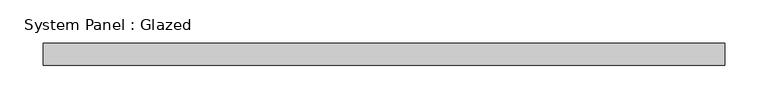
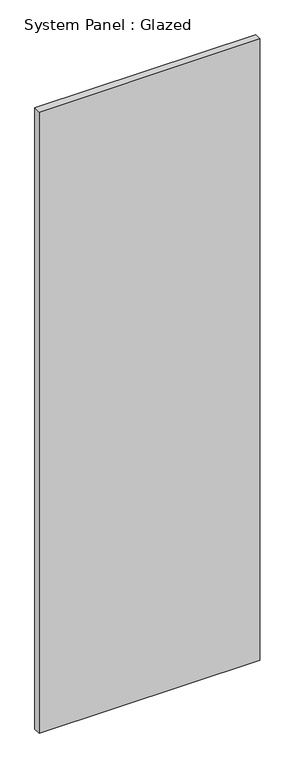
"""IFC4 building model written with IfcOpenShell, lengths in millimetres: plate geometry, System Panel : Glazed."""

from ifc_helpers import new_model, si_unit, origin, origin_with_axes, place, context, project, spatial, polyline, outline, extrude, source, transform, mapped, element, save


def system_panel_glazed_7e875482(model_context):
    return source(origin(), model_context, "Body", "SweptSolid", [
        extrude(outline(polyline([(393.7, 19.05), (-393.7, 19.05), (-393.7, 44.45), (393.7, 44.45), (393.7, 19.05)])), origin_with_axes(), (0.0, 0.0, 1.0), 2343.15),
    ])


if __name__ == "__main__":
    model = new_model("IFC4")
    model_context = context("Model", 3, world=origin())
    ifc_project = project(units=[si_unit("LENGTHUNIT", "METRE", prefix="MILLI")], contexts=[model_context])
    site = spatial("IfcSite", under=ifc_project)
    building = spatial("IfcBuilding", under=site)
    placement = place(None, origin())
    system_panel_glazed_shape = system_panel_glazed_7e875482(model_context)
    element("IfcPlate", 1, ObjectType="System Panel : Glazed", at=placement, inside=building, context=model_context, shape_type="MappedRepresentation", body=[
        mapped(system_panel_glazed_shape, transform((0.0, 0.0, 0.0), x_axis=(1.0, 0.0, 0.0), y_axis=(0.0, 1.0, 0.0), z_axis=(0.0, 0.0, 1.0))),
    ])
    save(model, "model.ifc")

# Revit data of these elements
# Type "System Panel : Glazed"
#   Construction Type Id = "GSP4R"
#   Analytic Construction = "1/8 in Pilkington single glazing"
#   Visual Light Transmittance = 0.9
#   Solar Heat Gain Coefficient = 0.86
#   Heat Transfer Coefficient (U) = 1.18115 BTU/(h·ft²·°F)
#   Define Thermal Properties by = 1
# Element 1 (IfcPlate, "System Panel : Glazed")
#   Materials on its faces: "Glass"
# Materials
#   "Glass": class "Glass", colour RGB 0 128 192, transparency 0.75, Description = "Soda Lime Glass", Cost = 0
